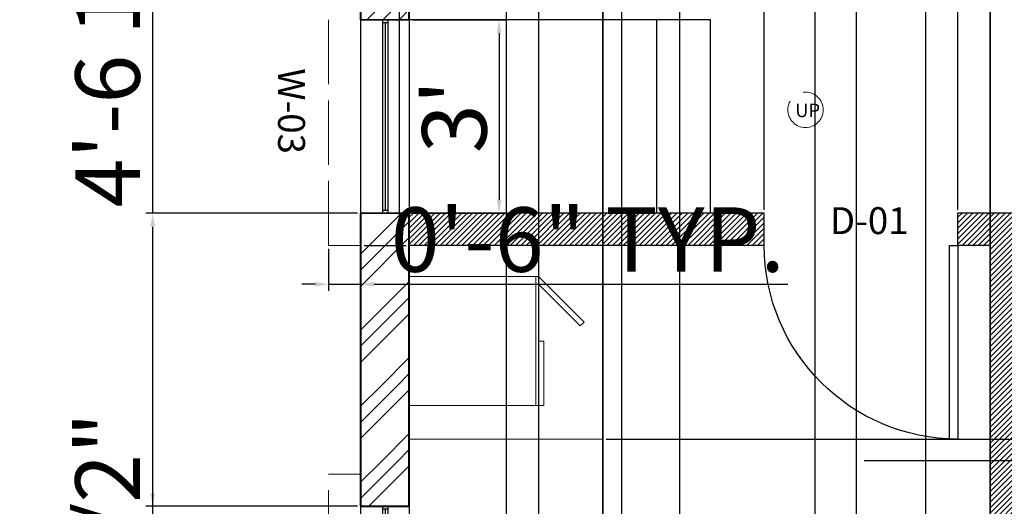
# Model space of a CAD drawing. Units: inches. Extents: x 2386 to 3029, y 792 to 1465.
# Tile 2 of 12: x 2408 to 2591, y 953 to 1044. Entities that reach past the tile are written whole.
import ezdxf

# ---------------------------------------------------------------- set-up
doc = ezdxf.new("R2010")
doc.units = ezdxf.units.IN
doc.linetypes.add('ACAD_ISO02W100', pattern=[15, 12, -3])
for name, color, linetype, lineweight in [('A-DIMS', 1, 'Continuous', 18), ('A-DOOR', 2, 'Continuous', 25), ('A-EQPM', 8, 'Continuous', 18), ('A-FLOR-CASE', 6, 'Continuous', 18), ('A-STAIR', 7, 'Continuous', 25), ('A-STAIR-PATH', 7, 'ACAD_ISO02W100', 18), ('A-TEXT', 4, 'Continuous', 25), ('A-WALL-EXT', 7, 'Continuous', 40), ('A-WALL-INT', 9, 'Continuous', 30), ('A-WALL-PATT', 9, 'Continuous', 13), ('A-WINDOW', 4, 'Continuous', 25), ('A-WINDOW-OVHD', 4, 'ACAD_ISO02W100', 18)]:
    doc.layers.add(name, color=color, linetype=linetype, lineweight=lineweight)
doc.styles.get("Standard").update_dxf_attribs({"font": 'arial.ttf'})
doc.dimstyles.new('ISO-25', dxfattribs={"dimtxt": 12, "dimasz": 2.5, "dimexe": 1.25, "dimexo": 0.625, "dimtad": 1, "dimlunit": 4, "dimtxsty": 'Standard', "dimcen": 2.5, "dimadec": 0, "dimazin": 0, "dimtfac": 1, "dimtmove": 0, "dimatfit": 3, "dimfxl": 1, "dimarcsym": 0})

# ---------------------------------------------------------------- blocks, each defined once
blk = doc.blocks.new('*U15')
for p, q in [((0, 0), (0, -6)), ((-40, 0), (-40, -6))]:
    blk.add_line(p, q)
blk.add_lwpolyline([(0, 0), (0, 40), (-1.75, 40), (-1.75, 0)], close=True)
blk.add_arc((0, 0), 40, 90, 180)
blk = doc.blocks.new('*D17')
at = {"layer": 'A-DIMS', "color": 0, "lineweight": -2, "transparency": 16777216}
for p, q in [((2480.82, 1043.95), (2498.14, 1043.95)), ((2496.89, 1041.45), (2496.89, 1010.45)), ((2480.82, 1007.95), (2498.14, 1007.95))]:
    blk.add_line(p, q, dxfattribs=at)
at = {"layer": 'A-DIMS', "color": 0, "transparency": 16777216}
for points in [[(2496.47, 1041.45), (2497.31, 1041.45), (2496.89, 1043.95)], [(2496.47, 1010.45), (2497.31, 1010.45), (2496.89, 1007.95)]]:
    blk.add_solid(points, dxfattribs=at)
at = {"layer": 'Defpoints', "color": 0, "transparency": 16777216}
for p in [(2480.19, 1043.95), (2480.19, 1007.95), (2496.89, 1007.95)]:
    blk.add_point(p, dxfattribs=at)
at = {"layer": 'A-DIMS', "color": 0, "transparency": 16777216, "insert": (2490.13, 1025.95), "char_height": 12, "attachment_point": 5, "rotation": 90}
blk.add_mtext("3'", dxfattribs=at)
blk = doc.blocks.new('REFRIGERATOR-24')
blk.add_line((23.5, 24), (23.5, 0))
for points in [[(24, 0), (0, 0), (0, 24), (24, 24)], [(24, 22.59), (31.78, 14.81), (32.49, 15.51), (24, 24), (24, 0), (25, 0), (25, 12), (24, 12)]]:
    blk.add_lwpolyline(points)
blk = doc.blocks.new('WINDOW-48IN')
for p, q in [((0, 9), (48, 9)), ((0, 0), (0, 9)), ((48, 9), (48, 0)), ((48, 5), (0, 5)), ((48, 4), (0, 4)), ((0.5, 4), (0.5, 5)), ((47.5, 4.5), (0.5, 4.5)), ((47.5, 5), (47.5, 4)), ((48, 0), (0, 0))]:
    blk.add_line(p, q)
blk = doc.blocks.new('WINDOW-HOOD-48IN')
for p, q in [((0, 0), (0, 6)), ((60, 6), (60, 0)), ((60, 0), (0, 0))]:
    blk.add_line(p, q)
blk = doc.blocks.new('WINDOW-36IN')
for p, q in [((0, 0), (0, 36)), ((4, 36), (4, 0)), ((4, 35.5), (5, 35.5)), ((4.5, 35.5), (4.5, 0.5)), ((5, 36), (5, 0)), ((9, 36), (9, 0)), ((5, 0.5), (4, 0.5))]:
    blk.add_line(p, q)
blk = doc.blocks.new('WINDOW-HOOD-36IN')
for p, q in [((0, 0), (0, 48)), ((0, 48), (6, 48)), ((6, 0), (0, 0))]:
    blk.add_line(p, q)
blk = doc.blocks.new('*D46')
at = {"layer": 'A-DIMS', "color": 0, "lineweight": -2, "transparency": 16777216}
for p, q in [((2478.39, 1049.95), (2478.39, 1225.86)), ((2471.82, 1049.95), (2479.64, 1049.95)), ((2478.39, 1004.45), (2478.39, 1047.45)), ((2471.82, 1001.95), (2479.64, 1001.95))]:
    blk.add_line(p, q, dxfattribs=at)
at = {"layer": 'A-DIMS', "color": 0, "transparency": 16777216}
for points in [[(2477.97, 1047.45), (2478.81, 1047.45), (2478.39, 1049.95)], [(2477.97, 1004.45), (2478.81, 1004.45), (2478.39, 1001.95)]]:
    blk.add_solid(points, dxfattribs=at)
at = {"layer": 'Defpoints', "color": 0, "transparency": 16777216}
for p in [(2471.19, 1049.95), (2478.39, 1049.95), (2471.19, 1001.95)]:
    blk.add_point(p, dxfattribs=at)
at = {"layer": 'A-DIMS', "color": 0, "transparency": 16777216, "insert": (2471.55, 1139.15), "char_height": 12, "attachment_point": 5, "rotation": 90}
blk.add_mtext('HOOD W-03 4\'-0" TYP.', dxfattribs=at)
blk = doc.blocks.new('*D47')
at = {"layer": 'A-DIMS', "color": 0, "lineweight": -2, "transparency": 16777216}
for p, q in [((2465.19, 1001.32), (2465.19, 993.5)), ((2471.19, 1001.32), (2471.19, 993.5)), ((2462.69, 994.75), (2460.19, 994.75)), ((2465.19, 994.75), (2471.19, 994.75)), ((2473.69, 994.75), (2550.59, 994.75))]:
    blk.add_line(p, q, dxfattribs=at)
at = {"layer": 'A-DIMS', "color": 0, "transparency": 16777216}
for points in [[(2462.69, 995.16), (2462.69, 994.33), (2465.19, 994.75)], [(2473.69, 995.16), (2473.69, 994.33), (2471.19, 994.75)]]:
    blk.add_solid(points, dxfattribs=at)
at = {"layer": 'Defpoints', "color": 0, "transparency": 16777216}
for p in [(2465.19, 1001.95), (2471.19, 1001.95), (2471.19, 994.75)]:
    blk.add_point(p, dxfattribs=at)
at = {"layer": 'A-DIMS', "color": 0, "transparency": 16777216, "insert": (2513.39, 1001.5), "char_height": 12, "attachment_point": 5}
blk.add_mtext('0\'-6" TYP.', dxfattribs=at)
blk = doc.blocks.new('*D57')
at = {"layer": 'A-DIMS', "color": 0, "lineweight": -2, "transparency": 16777216}
for p, q in [((2546.19, 1008.57), (2546.19, 1427.9)), ((2582.19, 1008.57), (2582.19, 1427.9)), ((2548.69, 1426.65), (2579.69, 1426.65))]:
    blk.add_line(p, q, dxfattribs=at)
at = {"layer": 'A-DIMS', "color": 0, "transparency": 16777216}
for points in [[(2548.69, 1427.06), (2548.69, 1426.23), (2546.19, 1426.65)], [(2579.69, 1427.06), (2579.69, 1426.23), (2582.19, 1426.65)]]:
    blk.add_solid(points, dxfattribs=at)
at = {"layer": 'Defpoints', "color": 0, "transparency": 16777216}
for p in [(2582.19, 1426.65), (2546.19, 1007.95), (2582.19, 1007.95)]:
    blk.add_point(p, dxfattribs=at)
at = {"layer": 'A-DIMS', "color": 0, "transparency": 16777216, "insert": (2564.19, 1433.4), "char_height": 12, "attachment_point": 5}
blk.add_mtext('3\'-0"', dxfattribs=at)
blk = doc.blocks.new('*D61')
at = {"layer": 'A-DIMS', "color": 0, "lineweight": -2, "transparency": 16777216}
for p, q in [((2432.49, 905.45), (2432.49, 969.54)), ((2470.57, 905.45), (2431.24, 905.45)), ((2432.49, 850.45), (2432.49, 902.95)), ((2470.57, 847.95), (2431.24, 847.95))]:
    blk.add_line(p, q, dxfattribs=at)
at = {"layer": 'A-DIMS', "color": 0, "transparency": 16777216}
for points in [[(2432.07, 902.95), (2432.91, 902.95), (2432.49, 905.45)], [(2432.07, 850.45), (2432.91, 850.45), (2432.49, 847.95)]]:
    blk.add_solid(points, dxfattribs=at)
at = {"layer": 'Defpoints', "color": 0, "transparency": 16777216}
for p in [(2432.49, 905.45), (2471.19, 905.45), (2471.19, 847.95)]:
    blk.add_point(p, dxfattribs=at)
at = {"layer": 'A-DIMS', "color": 0, "transparency": 16777216, "insert": (2425.66, 938.74), "char_height": 12, "attachment_point": 5, "rotation": 90}
blk.add_mtext('4\'-9 1/2"', dxfattribs=at)
blk = doc.blocks.new('*D62')
at = {"layer": 'A-DIMS', "color": 0, "lineweight": -2, "transparency": 16777216}
for p, q in [((2432.49, 1007.95), (2432.49, 1072.04)), ((2470.57, 1007.95), (2431.24, 1007.95)), ((2432.49, 955.95), (2432.49, 1005.45)), ((2470.57, 953.45), (2431.24, 953.45))]:
    blk.add_line(p, q, dxfattribs=at)
at = {"layer": 'A-DIMS', "color": 0, "transparency": 16777216}
for points in [[(2432.07, 1005.45), (2432.91, 1005.45), (2432.49, 1007.95)], [(2432.07, 955.95), (2432.91, 955.95), (2432.49, 953.45)]]:
    blk.add_solid(points, dxfattribs=at)
at = {"layer": 'Defpoints', "color": 0, "transparency": 16777216}
for p in [(2432.49, 1007.95), (2471.19, 1007.95), (2471.19, 953.45)]:
    blk.add_point(p, dxfattribs=at)
at = {"layer": 'A-DIMS', "color": 0, "transparency": 16777216, "insert": (2425.66, 1041.24), "char_height": 12, "attachment_point": 5, "rotation": 90}
blk.add_mtext('4\'-6 1/2"', dxfattribs=at)
blk = doc.blocks.new('*D73')
at = {"layer": 'A-DIMS', "color": 0, "lineweight": -2, "transparency": 16777216}
for p, q in [((2519.68, 889.97), (2519.68, 1427.9)), ((2555.68, 889.97), (2555.68, 1427.9)), ((2522.18, 1426.65), (2553.18, 1426.65))]:
    blk.add_line(p, q, dxfattribs=at)
at = {"layer": 'A-DIMS', "color": 0, "transparency": 16777216}
for points in [[(2522.18, 1427.06), (2522.18, 1426.23), (2519.68, 1426.65)], [(2553.18, 1427.06), (2553.18, 1426.23), (2555.68, 1426.65)]]:
    blk.add_solid(points, dxfattribs=at)
at = {"layer": 'Defpoints', "color": 0, "transparency": 16777216}
for p in [(2555.68, 1426.65), (2519.68, 889.35), (2555.68, 889.35)]:
    blk.add_point(p, dxfattribs=at)
at = {"layer": 'A-DIMS', "color": 0, "transparency": 16777216, "insert": (2537.68, 1433.4), "char_height": 12, "attachment_point": 5}
blk.add_mtext('3\'-0"', dxfattribs=at)
blk = doc.blocks.new('*D76')
at = {"layer": 'A-DIMS', "color": 0, "lineweight": -2, "transparency": 16777216}
for p, q in [((2480.19, 1174.77), (2480.19, 808)), ((2498.19, 1174.77), (2498.19, 808)), ((2482.69, 809.25), (2495.69, 809.25)), ((2498.19, 809.25), (2532.71, 809.25))]:
    blk.add_line(p, q, dxfattribs=at)
at = {"layer": 'A-DIMS', "color": 0, "transparency": 16777216}
for points in [[(2482.69, 809.66), (2482.69, 808.83), (2480.19, 809.25)], [(2495.69, 809.66), (2495.69, 808.83), (2498.19, 809.25)]]:
    blk.add_solid(points, dxfattribs=at)
at = {"layer": 'Defpoints', "color": 0, "transparency": 16777216}
for p in [(2480.19, 1175.39), (2498.19, 1175.39), (2498.19, 809.25)]:
    blk.add_point(p, dxfattribs=at)
at = {"layer": 'A-DIMS', "color": 0, "transparency": 16777216, "insert": (2516.7, 816), "char_height": 12, "attachment_point": 5}
blk.add_mtext('1\'-6"', dxfattribs=at)
blk = doc.blocks.new('*D77')
at = {"layer": 'A-DIMS', "color": 0, "lineweight": -2, "transparency": 16777216}
for p, q in [((2516.19, 1103.32), (2516.19, 808)), ((2576.19, 1103.32), (2576.19, 808)), ((2518.69, 809.25), (2573.69, 809.25))]:
    blk.add_line(p, q, dxfattribs=at)
at = {"layer": 'A-DIMS', "color": 0, "transparency": 16777216}
for points in [[(2518.69, 809.66), (2518.69, 808.83), (2516.19, 809.25)], [(2573.69, 809.66), (2573.69, 808.83), (2576.19, 809.25)]]:
    blk.add_solid(points, dxfattribs=at)
at = {"layer": 'Defpoints', "color": 0, "transparency": 16777216}
for p in [(2516.19, 1103.95), (2576.19, 1103.95), (2576.19, 809.25)]:
    blk.add_point(p, dxfattribs=at)
at = {"layer": 'A-DIMS', "color": 0, "transparency": 16777216, "insert": (2546.19, 816), "char_height": 12, "attachment_point": 5}
blk.add_mtext('5\'-0"', dxfattribs=at)
blk = doc.blocks.new('*D94')
at = {"layer": 'A-DIMS', "color": 0, "lineweight": -2, "transparency": 16777216}
for p, q in [((2504.19, 1205.32), (2504.19, 808)), ((2588.19, 1205.32), (2588.19, 808)), ((2506.69, 809.25), (2585.69, 809.25))]:
    blk.add_line(p, q, dxfattribs=at)
at = {"layer": 'A-DIMS', "color": 0, "transparency": 16777216}
for points in [[(2506.69, 809.66), (2506.69, 808.83), (2504.19, 809.25)], [(2585.69, 809.66), (2585.69, 808.83), (2588.19, 809.25)]]:
    blk.add_solid(points, dxfattribs=at)
at = {"layer": 'Defpoints', "color": 0, "transparency": 16777216}
for p in [(2504.19, 1205.95), (2588.19, 1205.95), (2588.19, 809.25)]:
    blk.add_point(p, dxfattribs=at)
at = {"layer": 'A-DIMS', "color": 0, "transparency": 16777216, "insert": (2546.19, 816), "char_height": 12, "attachment_point": 5}
blk.add_mtext('7\'-0"', dxfattribs=at)
blk = doc.blocks.new('*D96')
at = {"layer": 'A-DIMS', "color": 0, "lineweight": -2, "transparency": 16777216}
for p, q in [((2516.19, 893.57), (2516.19, 1427.9)), ((2588.19, 893.57), (2588.19, 1427.9)), ((2518.69, 1426.65), (2585.69, 1426.65))]:
    blk.add_line(p, q, dxfattribs=at)
at = {"layer": 'A-DIMS', "color": 0, "transparency": 16777216}
for points in [[(2518.69, 1427.06), (2518.69, 1426.23), (2516.19, 1426.65)], [(2585.69, 1427.06), (2585.69, 1426.23), (2588.19, 1426.65)]]:
    blk.add_solid(points, dxfattribs=at)
at = {"layer": 'Defpoints', "color": 0, "transparency": 16777216}
for p in [(2588.19, 1426.65), (2516.19, 892.95), (2588.19, 892.95)]:
    blk.add_point(p, dxfattribs=at)
at = {"layer": 'A-DIMS', "color": 0, "transparency": 16777216, "insert": (2552.19, 1433.4), "char_height": 12, "attachment_point": 5}
blk.add_mtext('6\'-0"', dxfattribs=at)
blk = doc.blocks.new('*D97')
at = {"layer": 'A-DIMS', "color": 0, "lineweight": -2, "transparency": 16777216}
for p, q in [((2516.82, 965.95), (2931.14, 965.95)), ((2929.89, 895.45), (2929.89, 963.45)), ((2516.82, 892.95), (2931.14, 892.95))]:
    blk.add_line(p, q, dxfattribs=at)
at = {"layer": 'A-DIMS', "color": 0, "transparency": 16777216}
for points in [[(2929.47, 963.45), (2930.31, 963.45), (2929.89, 965.95)], [(2929.47, 895.45), (2930.31, 895.45), (2929.89, 892.95)]]:
    blk.add_solid(points, dxfattribs=at)
at = {"layer": 'Defpoints', "color": 0, "transparency": 16777216}
for p in [(2516.19, 965.95), (2929.89, 965.95), (2516.19, 892.95)]:
    blk.add_point(p, dxfattribs=at)
at = {"layer": 'A-DIMS', "color": 0, "transparency": 16777216, "insert": (2923.14, 929.45), "char_height": 12, "attachment_point": 5, "rotation": 90}
blk.add_mtext('6\'-1"', dxfattribs=at)
blk = doc.blocks.new('*D99')
at = {"layer": 'A-DIMS', "color": 0, "lineweight": -2, "transparency": 16777216}
for p, q in [((2530.41, 1210.29), (2530.41, 808)), ((2563.26, 1210.63), (2563.26, 808)), ((2532.91, 809.25), (2560.76, 809.25)), ((2563.26, 809.25), (2599.11, 809.25))]:
    blk.add_line(p, q, dxfattribs=at)
at = {"layer": 'A-DIMS', "color": 0, "transparency": 16777216}
for points in [[(2532.91, 809.66), (2532.91, 808.83), (2530.41, 809.25)], [(2560.76, 809.66), (2560.76, 808.83), (2563.26, 809.25)]]:
    blk.add_solid(points, dxfattribs=at)
at = {"layer": 'Defpoints', "color": 0, "transparency": 16777216}
for p in [(2530.41, 1210.91), (2563.26, 1211.26), (2563.26, 809.25)]:
    blk.add_point(p, dxfattribs=at)
at = {"layer": 'A-DIMS', "color": 0, "transparency": 16777216, "insert": (2582.43, 816), "char_height": 12, "attachment_point": 5}
blk.add_mtext('2\'-9"', dxfattribs=at)
blk = doc.blocks.new('*D104')
at = {"layer": 'A-DIMS', "color": 0, "lineweight": -2, "transparency": 16777216}
for p, q in [((2564.73, 961.97), (2728.73, 961.97)), ((2854.11, 961.97), (2731.23, 961.97))]:
    blk.add_line(p, q, dxfattribs=at)
at = {"layer": 'A-DIMS', "color": 0, "transparency": 16777216}
blk.add_solid([(2731.23, 962.38), (2731.23, 961.55), (2728.73, 961.97)], dxfattribs=at)
at = {"layer": 'Defpoints', "color": 0, "transparency": 16777216}
for p in [(2564.73, 961.97), (2728.73, 961.97)]:
    blk.add_point(p, dxfattribs=at)
at = {"layer": 'A-DIMS', "color": 0, "transparency": 16777216, "insert": (2827.13, 968.72), "char_height": 12, "attachment_point": 5, "rotation": 359.9999}
blk.add_mtext('R13\'-8"', dxfattribs=at)

msp = doc.modelspace()

# ---------------------------------------------------------------- hatches: boundary and pattern name
at = {"layer": 'A-WALL-PATT'}
h = msp.add_hatch(dxfattribs=at)
h.set_pattern_fill('GOST_GROUND', color=256)
h.paths.add_polyline_path([(2480.19, 1276.948), (2471.19, 1276.948), (2471.19, 1211.948), (2480.19, 1211.948)])
h.paths.add_polyline_path([(2480.19, 1378.948), (2510.19, 1378.948), (2510.19, 1378.969), (2523.779, 1378.969), (2580.602, 1378.959), (2580.602, 1378.969), (2594.19, 1378.969), (2642.19, 1378.948), (2642.19, 1387.948), (2471.19, 1387.948), (2471.19, 1336.948), (2480.19, 1336.948)])
h.paths.add_polyline_path([(2891.19, 1387.948), (2666.19, 1387.948), (2666.19, 1378.948), (2882.19, 1378.948), (2882.19, 1355.948), (2891.19, 1355.948)])
h.paths.add_polyline_path([(2891.19, 1331.948), (2882.19, 1331.948), (2882.19, 1331.449), (2882.19, 1261.948), (2891.19, 1261.948)])
h.paths.add_polyline_path([(2891.19, 1201.948), (2882.19, 1201.948), (2882.19, 1189.948), (2882.19, 1159.948), (2882.19, 1117.948), (2891.19, 1117.948)])
h.paths.add_polyline_path([(2891.19, 1057.948), (2882.19, 1057.948), (2882.19, 856.948), (2882.19, 847.948), (2891.19, 847.948)])
h.paths.add_polyline_path([(2594.19, 856.948), (2558.19, 856.948), (2558.19, 847.948), (2594.19, 847.948)])
h.paths.add_polyline_path([(2510.19, 856.948), (2480.19, 856.948), (2480.19, 905.448), (2471.19, 905.448), (2471.19, 847.948), (2510.19, 847.948)])
h.paths.add_polyline_path([(2480.19, 1007.948), (2471.19, 1007.948), (2471.19, 953.448), (2480.19, 953.448)])
h.paths.add_polyline_path([(2480.19, 1103.948), (2471.19, 1103.948), (2471.19, 1043.948), (2480.19, 1043.948)])
h = msp.add_hatch(dxfattribs=at)
h.set_pattern_fill('JIS_WOOD', color=256)
h.paths.add_polyline_path([(2624.19, 1229.948), (2624.19, 1145.948), (2618.19, 1145.948), (2618.19, 1140.548), (2618.19, 1139.948), (2630.19, 1139.948), (2630.19, 1240.948), (2624.19, 1240.948), (2624.19, 1234.948), (2480.19, 1234.948), (2480.19, 1229.948)])
h.paths.add_polyline_path([(2582.19, 1139.948), (2582.19, 1145.948), (2480.19, 1145.948), (2480.19, 1139.948)], flags=17)
h.paths.add_polyline_path([(2480.19, 1007.948), (2480.19, 1001.948), (2546.19, 1001.948), (2546.19, 1007.348), (2546.19, 1007.948)])
h.paths.add_polyline_path([(2594.19, 1007.948), (2582.19, 1007.948), (2582.19, 1001.948), (2588.19, 1001.948), (2588.19, 856.948), (2594.19, 856.948), (2594.19, 914.948), (2606.19, 914.948), (2606.19, 920.948), (2594.19, 920.948)])
h.paths.add_polyline_path([(2738.19, 1015.948), (2882.19, 1015.948), (2882.19, 1021.948), (2738.19, 1021.948), (2738.19, 1111.948), (2732.19, 1111.948), (2732.19, 920.948), (2720.19, 920.948), (2720.19, 914.948), (2732.19, 914.948), (2732.19, 856.948), (2738.19, 856.948)])
h.paths.add_polyline_path([(2660.19, 914.948), (2660.19, 920.948), (2648.19, 920.948), (2648.19, 914.948)])
h.paths.add_polyline_path([(2738.19, 1159.948), (2738.19, 1165.948), (2737.59, 1165.948), (2732.19, 1165.948), (2732.19, 1147.948), (2737.59, 1147.948), (2738.19, 1147.948), (2738.19, 1153.948), (2882.19, 1153.948), (2882.19, 1159.948)])
h.paths.add_polyline_path([(2732.19, 1201.948), (2738.19, 1201.948), (2738.19, 1303.948), (2774.19, 1303.948), (2774.19, 1308.948), (2768.19, 1308.948), (2768.19, 1378.948), (2762.19, 1378.948), (2762.19, 1308.948), (2726.19, 1308.948), (2726.19, 1303.948), (2732.19, 1303.948)])
h.paths.add_polyline_path([(2696.19, 1303.948), (2696.19, 1308.948), (2630.19, 1308.948), (2630.19, 1378.948), (2624.19, 1378.948), (2624.19, 1276.948), (2630.19, 1276.948), (2630.19, 1303.948)])

# ---------------------------------------------------------------- linework, layer by layer
at = {"layer": 'A-FLOR-CASE'}
msp.add_lwpolyline([(2588.19, 892.948), (2516.19, 892.948), (2516.19, 965.948), (2480.19, 965.948)], dxfattribs=at)
at = {"layer": 'A-STAIR'}
for p, q in [((2516.19, 1007.948), (2516.19, 1103.948)), ((2536.19, 1043.948), (2471.19, 1043.948)), ((2526.19, 1007.948), (2526.19, 1043.948)), ((2536.19, 1007.948), (2536.19, 1043.948))]:
    msp.add_line(p, q, dxfattribs=at)
at = {"layer": 'A-STAIR-PATH'}
msp.add_lwpolyline([(2550.576, 1027.182, 0, 0, 0), (2507.381, 1027.182, 2, 0, 0), (2503.17, 1027.182, 0, 0, 0)], format="xyseb", dxfattribs=at)
msp.add_circle((2553.856, 1027.182), 3.28, dxfattribs=at)
at = {"layer": 'A-WALL-EXT'}
for p, q in [((2471.19, 1043.948), (2471.19, 1103.948)), ((2480.19, 1043.948), (2480.19, 1103.948)), ((2471.19, 953.448), (2471.19, 1007.948)), ((2480.19, 953.448), (2480.19, 1007.948)), ((2471.19, 953.448), (2480.19, 953.448)), ((2471.19, 953.448), (2480.19, 953.448)), ((2471.19, 953.448), (2480.19, 953.448))]:
    msp.add_line(p, q, dxfattribs=at)
at = {"layer": 'A-WALL-INT'}
for p, q in [((2546.19, 1007.948), (2471.19, 1007.948)), ((2546.19, 1001.948), (2546.19, 1007.948)), ((2594.19, 1007.948), (2582.19, 1007.948)), ((2582.19, 1001.948), (2582.19, 1007.948)), ((2546.19, 1001.948), (2480.19, 1001.948)), ((2588.19, 1001.948), (2582.19, 1001.948)), ((2588.19, 856.948), (2588.19, 1001.948))]:
    msp.add_line(p, q, dxfattribs=at)
at = {"layer": 'A-WINDOW'}
for p, q in [((2471.19, 1043.948), (2480.19, 1043.948)), ((2471.19, 1007.948), (2480.19, 1007.948))]:
    msp.add_line(p, q, dxfattribs=at)

# ---------------------------------------------------------------- block references
at = {"layer": 'A-DOOR', "xscale": -0.9, "yscale": 0.9, "zscale": 0.9, "rotation": 180}
msp.add_blockref('*U15', (2582.19, 1001.948), dxfattribs=at)
at = {"layer": 'A-EQPM'}
msp.add_blockref('REFRIGERATOR-24', (2480.19, 972.183), dxfattribs=at)
at = {"layer": 'A-WINDOW'}
msp.add_blockref('WINDOW-36IN', (2471.19, 1007.948), dxfattribs=at)
at = {"layer": 'A-WINDOW', "rotation": 89.99999999947651}
msp.add_blockref('WINDOW-48IN', (2480.19, 905.448), dxfattribs=at)
at = {"layer": 'A-WINDOW-OVHD'}
msp.add_blockref('WINDOW-HOOD-36IN', (2465.19, 1001.948), dxfattribs=at)
at = {"layer": 'A-WINDOW-OVHD', "rotation": 269.9999999991061}
msp.add_blockref('WINDOW-HOOD-48IN', (2465.19, 959.448), dxfattribs=at)

# ---------------------------------------------------------------- texts
at = {"layer": 'A-TEXT', "insert": (2460.804, 1034.906), "char_height": 5, "attachment_point": 1, "rotation": 270}
msp.add_mtext_dynamic_manual_height_columns('W-03', width=38.22215, gutter_width=12.5, heights=[0], dxfattribs=at)
at = {"layer": 'A-TEXT', "attachment_point": 1}
for s, width, insert, char_height in [('UP', 5.78227, (2551.946, 1028.324), 2.5), ('D-01', 38.22215, (2558.387, 1009.073), 5)]:
    msp.add_mtext_dynamic_manual_height_columns(s, width=width, gutter_width=12.5, heights=[0], dxfattribs=dict(at, insert=insert, char_height=char_height))

# ---------------------------------------------------------------- dimensions: what is measured, and where the dimension line sits
at = {"layer": 'A-DIMS'}
for base, p1, p2, picture, middle in [((2588.19, 1426.648), (2516.19, 892.948), (2588.19, 892.948), '*D96', (2552.19, 1433.4)), ((2555.676, 1426.648), (2519.676, 889.348), (2555.676, 889.348), '*D73', (2537.676, 1433.404)), ((2582.19, 1426.648), (2546.19, 1007.948), (2582.19, 1007.948), '*D57', (2564.19, 1433.404)), ((2563.257, 809.248), (2530.413, 1210.915), (2563.257, 1211.257), '*D99', (2582.434, 816)), ((2588.19, 809.248), (2504.19, 1205.948), (2588.19, 1205.948), '*D94', (2546.19, 816)), ((2498.19, 809.248), (2480.19, 1175.392), (2498.19, 1175.392), '*D76', (2516.7, 816)), ((2576.19, 809.248), (2516.19, 1103.948), (2576.19, 1103.948), '*D77', (2546.19, 816))]:
    dim = msp.add_linear_dim(base=base, p1=p1, p2=p2, dimstyle='ISO-25', override={"dimdec": 1, "dimlfac": 1, "dimrnd": 0, "dimzin": 1, "dimdsep": 46, "dimlunit": 4, "dimfrac": 2}, dxfattribs=at)
    dim.commit()
    dim.dimension.update_dxf_attribs({"geometry": picture, "text_midpoint": middle})
dim = msp.add_linear_dim(base=(2478.39, 1049.948), p1=(2471.19, 1001.948), p2=(2471.19, 1049.948), angle=90, text='HOOD W-03 <> TYP.', dimstyle='ISO-25', override={"dimdec": 1, "dimlfac": 1, "dimrnd": 0, "dimzin": 1, "dimdsep": 46, "dimlunit": 4, "dimfrac": 2}, dxfattribs=at)
dim.commit()
dim.dimension.update_dxf_attribs({"geometry": '*D46', "text_midpoint": (2471.552, 1139.152)})
for base, p1, p2, override, picture, middle in [((2432.49, 1007.948), (2471.19, 953.448), (2471.19, 1007.948), {"dimdec": 1, "dimlfac": 1, "dimrnd": 0, "dimzin": 1, "dimdsep": 46, "dimlunit": 4, "dimfrac": 2}, '*D62', (2425.66, 1041.245)), ((2496.891, 1007.948), (2480.19, 1043.948), (2480.19, 1007.948), {"dimclrd": 0, "dimclre": 0, "dimclrt": 0}, '*D17', (2490.135, 1025.948)), ((2432.49, 905.448), (2471.19, 847.948), (2471.19, 905.448), {"dimdec": 1, "dimlfac": 1, "dimrnd": 0, "dimzin": 1, "dimdsep": 46, "dimlunit": 4, "dimfrac": 2}, '*D61', (2425.66, 938.745)), ((2929.89, 965.948), (2516.19, 892.948), (2516.19, 965.948), {"dimdec": 1, "dimlfac": 1, "dimrnd": 0, "dimzin": 1, "dimdsep": 46, "dimlunit": 4, "dimfrac": 2}, '*D97', (2923.138, 929.448))]:
    dim = msp.add_linear_dim(base=base, p1=p1, p2=p2, angle=90, dimstyle='ISO-25', override=override, dxfattribs=at)
    dim.commit()
    dim.dimension.update_dxf_attribs({"geometry": picture, "text_midpoint": middle})
dim = msp.add_linear_dim(base=(2471.19, 994.748), p1=(2465.19, 1001.948), p2=(2471.19, 1001.948), text='<> TYP.', dimstyle='ISO-25', override={"dimdec": 1, "dimlfac": 1, "dimrnd": 0, "dimzin": 1, "dimdsep": 46, "dimlunit": 4, "dimfrac": 2}, dxfattribs=at)
dim.commit()
dim.dimension.update_dxf_attribs({"geometry": '*D47', "text_midpoint": (2513.388, 1001.5)})
dim = msp.add_radius_dim(center=(2564.73, 961.967), mpoint=(2728.73, 961.967), dimstyle='ISO-25', override={"dimdec": 1, "dimlfac": 1, "dimrnd": 0, "dimzin": 1, "dimdsep": 46, "dimlunit": 4, "dimfrac": 2}, dxfattribs=at)
dim.commit()
dim.dimension.update_dxf_attribs({"geometry": '*D104', "text_midpoint": (2827.13, 961.967), "dimtype": 164})

doc.saveas('drawing.dxf')
